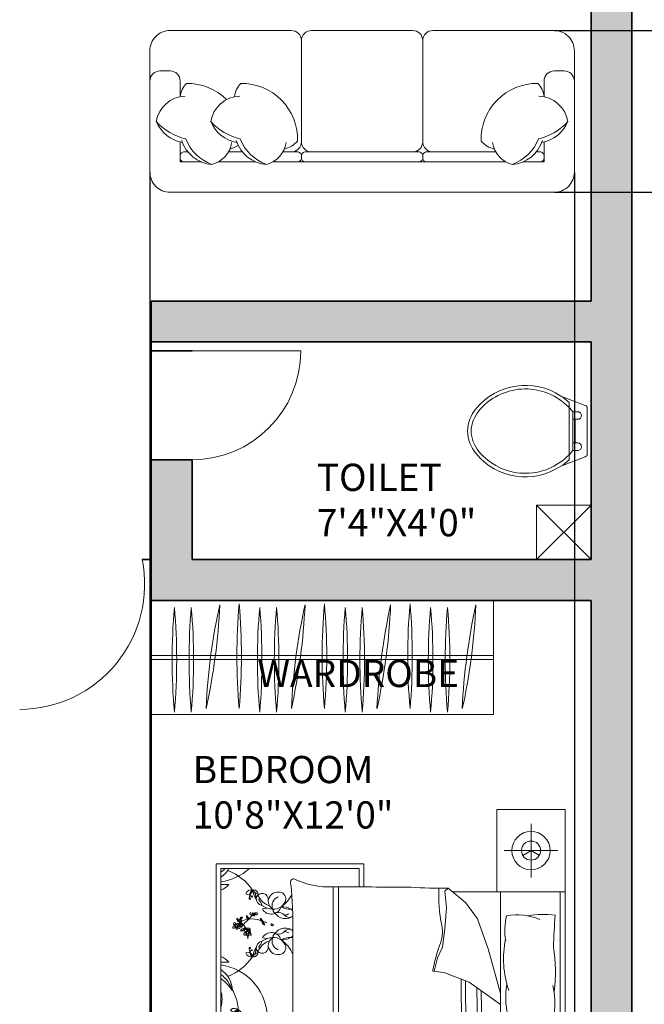
# Model space of a CAD drawing. Units: inches. Extents: x 37 to 706, y -568 to 110.
# Tile 8 of 24: x 223 to 361, y -450 to -233. Entities that reach past the tile are written whole.
import ezdxf

# ---------------------------------------------------------------- set-up
doc = ezdxf.new("R2010")
doc.units = ezdxf.units.IN
doc.header["$MEASUREMENT"] = 0
for name, color, linetype, lineweight in [('A-ANNO-DIMS', 2, 'Continuous', 18), ('A-ANNO-TEXT', 7, 'Continuous', 18), ('A-AREA-IDEN', 7, 'Continuous', 18), ('A-DOOR', 4, 'Continuous', 18), ('A-FLOR-CASE', 9, 'Continuous', 18), ('A-FLOR-FIXT', 9, 'Continuous', 18), ('A-FLOR-OPEN', 8, 'Continuous', 13), ('A-FURN', 8, 'Continuous', 13), ('A-WALL', 7, 'Continuous', 35), ('A-WALL-PATT', 252, 'Continuous', 13)]:
    doc.layers.add(name, color=color, linetype=linetype, lineweight=lineweight)
doc.styles.get("Standard").update_dxf_attribs({"font": 'arial.ttf'})
doc.dimstyles.get("Standard").update_dxf_attribs({"dimtxt": 0.18, "dimasz": 0.18, "dimexe": 0.18, "dimexo": 0.0625, "dimgap": 0.09, "dimtad": 0, "dimtih": 1, "dimtoh": 1, "dimdec": 0, "dimzin": 0, "dimdsep": 46, "dimlunit": 3, "dimtxsty": 'Standard', "dimcen": 0.09, "dimadec": 0, "dimazin": 0, "dimtfac": 1, "dimtdec": 0, "dimtofl": 0, "dimtmove": 0, "dimatfit": 3, "dimfxl": 1, "dimtolj": 1, "dimtzin": 0, "dimarcsym": 0})

# ---------------------------------------------------------------- blocks, each defined once
blk = doc.blocks.new('WARDROBE-DOUBLE')
for p, q in [((75.49, 25.16), (0, 25.16)), ((0, 25.16), (0, 0)), ((75.49, 25.16), (75.49, 0)), ((75.49, 13), (0, 13)), ((75.49, 12.16), (0, 12.16)), ((75.49, 0), (0, 0))]:
    blk.add_line(p, q)
for centre, start, end in [((-117.16, 29.99), 347.508, 357.5023), ((144.38, -4.42), 167.508, 177.5023), ((151.29, 12.89), 175.0028, 184.9972), ((-112.5, 12.89), 355.0028, 4.9972), ((-98.35, 29.99), 347.508, 357.5023), ((163.19, -4.42), 167.508, 177.5023), ((170.1, 12.89), 175.0028, 184.9972), ((-93.69, 12.89), 355.0028, 4.9972), ((182.06, -4.42), 167.508, 177.5023), ((-79.47, 29.99), 347.508, 357.5023), ((188.97, 12.89), 175.0028, 184.9972), ((-74.82, 12.89), 355.0028, 4.9972), ((200.87, -4.42), 167.508, 177.5023), ((-60.66, 29.99), 347.508, 357.5023), ((137.01, 12.08), 175.0028, 184.9972), ((-126.78, 12.08), 355.0028, 4.9972), ((140.74, 12.08), 175.0028, 184.9972), ((-123.05, 12.08), 355.0028, 4.9972), ((155.82, 12.08), 175.0028, 184.9972), ((-107.97, 12.08), 355.0028, 4.9972), ((159.55, 12.08), 175.0028, 184.9972), ((-104.24, 12.08), 355.0028, 4.9972), ((174.7, 12.08), 175.0028, 184.9972), ((-89.09, 12.08), 355.0028, 4.9972), ((178.43, 12.08), 175.0028, 184.9972), ((-85.36, 12.08), 355.0028, 4.9972), ((193.51, 12.08), 175.0028, 184.9972), ((-70.28, 12.08), 355.0028, 4.9972), ((197.24, 12.08), 175.0028, 184.9972), ((-66.55, 12.08), 355.0028, 4.9972)]:
    blk.add_arc(centre, 132.4, start, end)
blk = doc.blocks.new('WC-PLAN')
for p, q in [((22.41, 16.39), (22.41, 15.28)), ((22.41, 15.28), (22.41, 10.09)), ((22.41, 4.89), (22.41, 10.09)), ((22.41, 4.89), (22.41, 3.79))]:
    blk.add_line(p, q)
for points in [[(20.6, 17.82, 0.383919), (1.9, 15.05, 0.163732), (0, 10.09, 0.359733)], [(21.87, 15.81, 0.431639), (2.51, 14.55, 0.162618), (0.79, 10.09, 0.470877)], [(22.41, 16.39, 0.040937), (20.6, 17.82, 0.163732)], [(26.41, 10.09), (26.41, 15.13, 0.31031), (25.98, 15.75), (20.6, 17.82, 0.209071)], [(22.41, 15.28, 0.014165), (21.87, 15.81, 0.162618)], [(23.21, 14.37, 0.022712), (22.41, 15.28, 0.162618)], [(23.21, 10.09), (23.21, 14.37, 0.022712)], [(23.21, 14.37), (24.32, 14.37, -1), (24.32, 12.69), (23.74, 12.69)], [(20.6, 2.36, -0.383919), (1.9, 5.12, -0.163732), (0, 10.09, -0.359733)], [(22.41, 4.89, -0.448546), (2.51, 5.63, -0.162618), (0.79, 10.09, -0.470877)], [(26.41, 10.09), (26.41, 5.05, -0.31031), (25.98, 4.43), (20.6, 2.36, -0.209071)], [(23.21, 10.09), (23.21, 5.8, -0.476108)], [(23.21, 5.8), (24.32, 5.8, 1), (24.32, 7.49), (23.74, 7.49)], [(23.21, 5.8, -0.022712), (22.41, 4.89, -0.162618)], [(22.41, 3.79, -0.040937), (20.6, 2.36, -0.163732)]]:
    blk.add_lwpolyline(points, format="xyb")
for points in [[(23.74, 12.69), (23.21, 12.69)], [(23.74, 7.49), (23.74, 12.69)], [(23.74, 7.49), (23.21, 7.49)]]:
    blk.add_lwpolyline(points)
blk = doc.blocks.new('BED-DOUBLE-WITH-NIGHTSTANDS')
for p, q in [((77.02, 90.57), (77.02, 0)), ((69.47, 75.59), (69.47, 87.43)), ((63.56, 81.51), (75.39, 81.51)), ((0, 78.61), (32.62, 78.61)), ((0, 12.59), (0, 78.61)), ((32.62, 78.61), (32.62, 73.49)), ((1.05, 77.56), (1.05, 13.64)), ((31.58, 77.56), (1.05, 77.56)), ((31.58, 73.49), (31.58, 77.56)), ((25.85, 17.62), (25.85, 73.5)), ((26.98, 17.7), (26.98, 73.5)), ((50.48, 72.53), (51.22, 73.26)), ((50.85, 68.86), (50.48, 72.53)), ((51.22, 73.26), (55.07, 69.96)), ((77.02, 72.45), (52.16, 72.45)), ((62.71, 72.45), (62.71, 18.11)), ((75.86, 18.11), (75.86, 72.45)), ((55.07, 69.96), (57.63, 66.48)), ((10.23, 68.64), (11.25, 68.84)), ((50.48, 64.28), (50.85, 68.86)), ((57.63, 66.48), (60.02, 59.87)), ((16.95, 26.9), (16.95, 63.67)), ((49.93, 60.24), (50.48, 64.28)), ((10.23, 62.31), (11.25, 62.11)), ((48.83, 57.86), (49.93, 60.24)), ((60.02, 59.87), (62.71, 50)), ((48.1, 54.92), (48.83, 57.86)), ((50.48, 54.55), (48.1, 54.92)), ((55.8, 52.54), (50.48, 54.55)), ((54.24, 18.43), (54.09, 53.18)), ((55.17, 18.44), (55.03, 52.83)), ((62.71, 47.57), (55.8, 52.54)), ((58.02, 18.39), (57.55, 51.28)), ((58.95, 18.36), (58.49, 50.6)), ((10.23, 28.89), (11.25, 29.09)), ((10.23, 22.56), (11.25, 22.36)), ((31.58, 13.64), (31.58, 17.63)), ((32.62, 17.61), (32.62, 12.59)), ((1.05, 13.64), (31.58, 13.64)), ((69.47, 14.97), (69.47, 3.14)), ((32.62, 12.59), (0, 12.59))]:
    blk.add_line(p, q)
for points in [[(61.93, 72.45), (61.93, 90.57), (77.02, 90.57)], [(69.47, 81.51), (67.64, 80.45)], [(69.47, 81.51), (71.3, 80.45)], [(77.02, 18.11), (61.93, 18.11), (61.93, 0), (77.02, 0)], [(69.47, 9.06), (67.64, 10.11)], [(69.47, 9.06), (71.3, 10.11)]]:
    blk.add_lwpolyline(points)
for points in [[(42.92, 73.45, 0.001242), (25.74, 73.5, -0.127202), (17.18, 75.31)], [(74.76, 67.25, 0.074897), (68.85, 67.14, -0.472817)], [(68.52, 45.71, 0.14099), (74.55, 45.53, 0.235245)], [(68.52, 41.84, -0.14099), (74.55, 42.02, -0.235245)], [(74.76, 23.32, -0.074897), (68.85, 23.42, 0.472817)], [(27.69, 17.73, 0.056112), (22.71, 17.07, 0.095341), (17.91, 15.8)]]:
    blk.add_lwpolyline(points, format="xyb")
for centre, radius in [((69.47, 81.51), 4.23), ((69.47, 81.51), 2.11), ((4.52, 64.91), 0.231), ((6.95, 63.41), 0.231), ((4.52, 26.28), 0.231), ((6.95, 27.79), 0.231), ((69.47, 9.06), 4.23), ((69.47, 9.06), 2.11)]:
    blk.add_circle(centre, radius)
for centre, radius, start, end in [((-3.2, 82.51), 7.18, 306.3036, 316.4814), ((-2.13, 80.43), 5.76, 303.4617, 330.1116), ((-0.54, 86.37), 11.83, 277.745, 311.8856), ((-1.71, 66.13), 11.83, 34.3865, 68.5908), ((-0.79, 77.21), 4.81, 292.5547, 318.9546), ((1.79, 90.38), 16.36, 267.4081, 273.6519), ((17.23, 74.48), 0.836, 93.98, 207.3412), ((-77.32, 64.75), 94.28, 359.3433, 5.6887), ((7.77, 71.53), 1.31, 77.7115, 159.0387), ((7.06, 72.84), 0.988, 238.4633, 358.2869), ((10.3, 70.85), 2.99, 138.8402, 177.9352), ((8.5, 71.96), 0.967, 117.6827, 223.7762), ((8.28, 71.86), 0.98, 2.9516, 103.728), ((16.12, 74.61), 8.27, 192.5173, 207.1824), ((6.95, 71.3), 1.87, 345.4653, 54.2343), ((9.77, 73.87), 2.02, 211.3827, 255.2969), ((10.16, 70.71), 1.36, 350.264, 160.8688), ((8.69, 70.99), 0.833, 333.9755, 53.2681), ((13.65, 70.21), 2.16, 84.9449, 172.8857), ((13.86, 70.84), 1.53, 354.4856, 91.0538), ((10.57, 74.83), 6.85, 303.6671, 333.2997), ((48.97, 156.3), 83.07, 265.8294, 271.553), ((83.29, 71.71), 34.18, 177.4519, 191.3392), ((7.46, 70.95), 0.147, 177.9352, 11.4834), ((7.53, 70.96), 0.0713, 11.4834, 127.9409), ((7.89, 71.38), 0.128, 223.7762, 159.7183), ((10.57, 71.04), 1.7, 175.969, 254.3045), ((8.31, 69.21), 1.81, 6.1662, 51.5825), ((13.15, 73.4), 4.28, 211.2614, 251.7045), ((14.13, 70.59), 2.63, 182.3591, 234.0401), ((14.47, 69.36), 2.1, 111.5819, 201.4221), ((12.73, 71.31), 2.72, 265.2933, 346.921), ((1.34, 72.69), 8.6, 313.1541, 322.0459), ((7.66, 67.53), 0.177, 142.4737, 265.053), ((7.89, 67.56), 0.381, 127.7621, 169.0403), ((7.69, 67.89), 0.536, 265.053, 338.3618), ((8.4, 67.15), 0.7, 113.4276, 137.6104), ((8.32, 67.88), 0.231, 183.2768, 356.7232), ((8.49, 67.46), 0.377, 139.7889, 227.6792), ((8.37, 67.33), 0.199, 227.6792, 350.3487), ((7.6, 67.46), 0.755, 353.0852, 15.7171), ((8.1, 67.37), 0.477, 350.3487, 43.6538), ((8.98, 67.87), 0.555, 198.7263, 262.5032), ((8.54, 67.61), 0.22, 1.1081, 91.8675), ((8.68, 67.56), 0.385, 11.5637, 52.6358), ((8.95, 67.49), 0.178, 255.2356, 54.9248), ((12.81, 73.44), 4.86, 236.2883, 266.5076), ((12.18, 69.76), 2.25, 209.9085, 343.1337), ((13.13, 68.34), 0.562, 167.3041, 285.1471), ((14.65, 65.65), 3.49, 122.7011, 126.3445), ((15.31, 69.41), 2.89, 199.2822, 299.1751), ((13.76, 66), 1.86, 41.5653, 105.1471), ((16.28, 72.32), 3.75, 238.8218, 279.1554), ((14.65, 65.65), 3.49, 55.785, 94.7304), ((14.78, 69.85), 2.6, 277.436, 299.9149), ((15.95, 67.67), 1.09, 30.0293, 52.325), ((66.47, 55.71), 11.67, 65.1316, 101.7583), ((4.34, 65.38), 0.455, 157.4086, 261.4386), ((4.09, 65.4), 0.229, 58.0499, 135.6268), ((4.32, 65.26), 0.153, 172.906, 277.132), ((3.82, 64.98), 0.727, 14.7558, 58.0499), ((4.84, 65.17), 0.315, 36.1046, 181.4281), ((4.85, 66.4), 0.258, 124.3538, 214.3923), ((5.23, 66.36), 0.6, 190.3057, 287.1958), ((4.66, 65.42), 0.317, 270.0645, 331.1507), ((5.41, 66.58), 0.697, 176.9701, 248.2913), ((10.38, 70.25), 6.74, 212.6784, 216.3746), ((4.92, 65.2), 0.226, 263.7526, 41.7054), ((5.17, 66.41), 0.267, 216.3746, 291.7548), ((7.53, 62.67), 3.76, 124.0033, 132.4917), ((3.66, 62.2), 4.02, 63.7819, 68.2913), ((5.81, 65.29), 0.639, 128.3208, 208.8162), ((5.81, 66.23), 0.6, 122.8155, 187.3992), ((5.34, 65.98), 0.201, 289.3605, 111.7548), ((5.49, 65.98), 0.201, 221.8703, 44.2646), ((6.41, 65.39), 1.05, 157.2305, 229.0635), ((6.07, 66.15), 0.697, 109.4799, 177.6828), ((6.05, 65.74), 0.619, 174.4544, 220.6188), ((2.53, 62.29), 4.51, 30.544, 49.818), ((5.7, 66.59), 0.258, 56.8636, 146.9021), ((5.83, 66.31), 0.267, 148.8844, 224.2646), ((5.02, 64.86), 0.744, 340.0041, 40.6188), ((11.37, 62.96), 6.74, 145.1882, 148.8844), ((7.53, 62.67), 3.76, 94.756, 119.2041), ((15.54, 57.26), 12.37, 132.2412, 142.1744), ((9.29, 67.11), 2.55, 178.3264, 187.1302), ((6.53, 66.75), 0.476, 11.3256, 64.4621), ((8.15, 67.44), 1.43, 190.2588, 210.656), ((7.19, 66.85), 0.435, 188.3432, 274.2869), ((7.57, 67.09), 0.759, 210.656, 242.6341), ((8.14, 67.75), 1.46, 218.2101, 226.3071), ((7.07, 66.52), 0.185, 325.7657, 67.4417), ((7.72, 58.94), 7.5, 73.5842, 93.8277), ((12.34, 66.57), 2.55, 178.3264, 187.1302), ((9.58, 66.21), 0.476, 11.3256, 64.4621), ((11.19, 66.9), 1.43, 190.2588, 210.656), ((10.23, 66.31), 0.435, 188.3432, 274.2869), ((10.61, 66.55), 0.759, 210.656, 242.6341), ((11.19, 67.21), 1.46, 218.2101, 226.3071), ((10.11, 65.98), 0.185, 325.7657, 67.4417), ((10.63, 65.65), 0.435, 147.5332, 233.4768), ((11.02, 65.87), 0.759, 179.1859, 211.164), ((10.28, 65.7), 0.185, 354.3784, 96.0543), ((7.72, 58.94), 7.5, 63.0032, 69.8941), ((11.6, 66.22), 1.43, 211.164, 231.5612), ((11.85, 67.38), 2.55, 234.6898, 243.4936), ((11.87, 66.07), 1.46, 195.5129, 203.6099), ((10.23, 65.12), 0.476, 357.3579, 50.4944), ((12.28, 65.21), 0.175, 12.7051, 190.4384), ((12.38, 65.23), 0.284, 190.4384, 10.4136), ((16.16, 68.13), 1.36, 221.5653, 293.8354), ((15.95, 67.67), 1.09, 314.4517, 333.558), ((75.82, 64.02), 12.14, 165.1039, 191.0369), ((936.66, 17.33), 863.34, 176.68521, 177.14978), ((3.86, 64.56), 0.177, 142.4737, 265.053), ((4.09, 64.6), 0.381, 61.2196, 169.0403), ((3.89, 64.92), 0.536, 265.053, 338.3618), ((4.6, 64.19), 0.7, 113.4276, 137.6104), ((4.69, 64.5), 0.377, 139.7889, 227.6792), ((4.57, 64.37), 0.199, 227.6792, 350.3487), ((3.8, 64.5), 0.755, 353.0852, 15.7171), ((4.29, 64.41), 0.477, 350.3487, 43.6538), ((5.18, 64.9), 0.555, 198.7263, 262.5032), ((4.93, 65.34), 0.363, 221.8413, 265.7877), ((4.74, 64.65), 0.22, 1.1081, 91.8675), ((4.88, 64.6), 0.385, 11.5637, 86.365), ((5.15, 64.53), 0.178, 255.2356, 54.9248), ((5.92, 65.34), 0.764, 207.7043, 254.3516), ((5.43, 64.9), 1.05, 270.278, 342.111), ((6.13, 63.58), 0.744, 98.7227, 159.3375), ((5.75, 64.54), 0.764, 244.9899, 291.6373), ((5.92, 64.93), 0.619, 278.7227, 324.8872), ((5.81, 64.43), 0.639, 290.5253, 358.5375), ((6.29, 63.06), 0.177, 142.4737, 265.053), ((6.52, 63.09), 0.381, 61.2196, 169.0403), ((6.32, 63.41), 0.536, 265.053, 338.3618), ((6.77, 63.88), 0.455, 157.4086, 261.4386), ((6.52, 63.89), 0.229, 58.0499, 135.6268), ((7.06, 64.61), 0.639, 182.8499, 266.1226), ((6.81, 65.06), 0.619, 231.7607, 277.9252), ((7.29, 65.17), 1.05, 214.5369, 286.3699), ((7.03, 62.68), 0.7, 113.4276, 137.6104), ((6.76, 63.75), 0.153, 172.906, 277.132), ((6.25, 63.47), 0.727, 14.7558, 58.0499), ((2.53, 62.29), 4.51, 23.0501, 23.8477), ((7.12, 62.99), 0.377, 139.7889, 227.6792), ((7, 63.71), 0.744, 37.3105, 97.9252), ((7.27, 63.66), 0.315, 36.1046, 181.4281), ((6.23, 62.99), 0.755, 353.0852, 15.7171), ((7.08, 64.73), 0.764, 265.0106, 311.658), ((6.72, 62.9), 0.477, 350.3487, 43.6538), ((7.61, 63.4), 0.555, 198.7263, 262.5032), ((7.09, 63.91), 0.317, 270.0645, 331.1507), ((7.36, 63.83), 0.363, 221.8413, 265.7877), ((7.17, 63.14), 0.22, 1.1081, 91.8675), ((7.36, 63.7), 0.226, 263.7526, 41.7054), ((7.31, 63.09), 0.385, 11.5637, 86.365), ((7.58, 63.02), 0.178, 255.2356, 54.9248), ((12.18, 61.19), 2.25, 16.8663, 150.0915), ((13.13, 62.61), 0.562, 74.8529, 192.6959), ((15.31, 61.54), 2.89, 60.8249, 160.7178), ((13.76, 64.95), 1.86, 254.8529, 318.4347), ((14.78, 61.1), 2.6, 60.0851, 82.564), ((16.16, 62.82), 1.36, 66.1646, 138.4347), ((15.95, 63.28), 1.09, 23.229, 45.5483), ((42.55, 63.54), 7.37, 336.2616, 11.3392), ((7, 62.86), 0.199, 227.6792, 350.3487), ((2.53, 62.29), 4.51, 357.1071, 4.7585), ((10.57, 59.91), 1.7, 105.6955, 184.031), ((8.31, 61.74), 1.81, 308.4175, 353.8338), ((13.15, 57.54), 4.28, 108.2955, 148.7386), ((12.81, 57.5), 4.86, 93.4924, 123.7117), ((14.13, 60.36), 2.63, 125.9599, 177.6409), ((14.47, 61.59), 2.1, 158.5779, 248.4181), ((12.73, 59.64), 2.72, 13.079, 94.7067), ((14.65, 65.3), 3.49, 233.6555, 237.2989), ((16.28, 58.63), 3.75, 79.7133, 121.1782), ((14.65, 65.3), 3.49, 265.2696, 304.215), ((10.57, 56.11), 6.85, 21.4941, 56.3329), ((15.95, 63.28), 1.09, 307.675, 336.7144), ((84.45, 57.63), 21.05, 168.0397, 199.2615), ((7.06, 58.1), 0.988, 1.7131, 121.5367), ((7.77, 59.41), 1.31, 200.9613, 282.2885), ((7.46, 60), 0.147, 348.5166, 182.0648), ((10.3, 60.1), 2.99, 182.0648, 221.1598), ((7.53, 59.98), 0.0713, 232.0591, 348.5166), ((8.5, 58.99), 0.967, 136.2238, 242.3173), ((7.94, 59.56), 0.0771, 200.2667, 136.2271), ((6.95, 59.65), 1.87, 305.7657, 14.5347), ((16.12, 56.34), 8.27, 152.8176, 167.4827), ((8.28, 59.09), 0.98, 256.272, 357.0484), ((9.77, 57.08), 2.02, 104.7031, 148.6173), ((10.16, 60.24), 1.36, 199.1312, 9.736), ((8.69, 59.96), 0.833, 306.7319, 26.0245), ((13.65, 60.74), 2.16, 187.1143, 275.0551), ((13.86, 60.11), 1.53, 268.9462, 5.5144), ((82.33, 48.63), 35.12, 160.1194, 169.3383), ((41.99, 54.84), 32.85, 352.2196, 9.497), ((-0.79, 53.74), 4.81, 41.0454, 67.4453), ((1.79, 40.57), 16.36, 86.3481, 92.5919), ((-1.71, 64.81), 11.83, 291.4092, 325.6135), ((-0.54, 44.58), 11.83, 4.4623, 82.255), ((-2.13, 50.51), 5.76, 1.272, 56.5383), ((48.03, 55.13), 0.219, 178.8623, 289.7536), ((-3.2, 48.44), 7.18, 17.8504, 53.6964), ((-5.22, 44.66), 10.68, 34.0123, 54.053), ((-5.17, 48.79), 6.5, 343.5431, 17.0202), ((-6.88, 45.48), 11.83, 4.4623, 27.4146), ((79.85, 49.11), 15.97, 169.8617, 193.6238), ((58.59, 47.9), 16.14, 351.5249, 13.96), ((-8.52, 46.22), 9.62, 4.3787, 5.6357), ((-15.11, 41.15), 17.18, 19.7217, 19.9028), ((4.03, 45.43), 1.31, 47.7873, 129.1145), ((4.07, 46.92), 0.988, 208.5391, 328.3627), ((5.88, 43.58), 2.99, 108.9159, 148.011), ((4.87, 45.44), 0.967, 87.7585, 193.852), ((12.81, 43.93), 8.27, 162.593, 177.2582), ((3.21, 45.64), 1.87, 315.5411, 24.3101), ((6.93, 46.46), 2.02, 181.4585, 225.3727), ((4.64, 45.46), 0.98, 333.0274, 73.8037), ((10.37, 44.53), 1.31, 47.7873, 129.1145), ((65.49, 56.38), 11.1, 264.0129, 285.8293), ((3.47, 45.08), 0.147, 148.011, 341.5592), ((3.54, 45.06), 0.0713, 341.5592, 98.0167), ((4.06, 45.24), 0.128, 193.852, 129.9245), ((12.81, 44.25), 8.27, 182.7418, 197.407), ((3.21, 42.54), 1.87, 335.6899, 44.4589), ((10.41, 46.02), 0.988, 208.5391, 328.3627), ((9.8, 44.18), 0.147, 148.011, 341.5592), ((9.8, 44), 0.147, 18.4408, 211.989), ((12.22, 42.67), 2.99, 108.9159, 148.011), ((12.22, 45.51), 2.99, 211.989, 251.0841), ((9.88, 44.15), 0.0713, 341.5592, 98.0167), ((9.88, 44.03), 0.0713, 261.9833, 18.4408), ((11.21, 44.53), 0.967, 87.7585, 193.852), ((11.21, 43.65), 0.967, 166.148, 272.2415), ((10.39, 44.33), 0.128, 193.852, 129.9245), ((10.44, 43.86), 0.0771, 230.1909, 166.0209), ((9.54, 44.73), 1.87, 315.5411, 24.3101), ((19.14, 43.02), 8.27, 162.593, 177.2582), ((9.54, 43.45), 1.87, 335.6899, 44.4589), ((19.14, 45.16), 8.27, 182.7418, 197.407), ((10.97, 44.56), 0.98, 333.0274, 73.8037), ((13.27, 45.55), 2.02, 181.4585, 225.3727), ((10.97, 43.62), 0.98, 286.1963, 26.9726), ((13.27, 42.63), 2.02, 134.6273, 178.5415), ((2.19, 43.98), 9.15, 262.8636, 351.8197), ((4.07, 41.26), 0.988, 31.6373, 151.4609), ((4.03, 42.75), 1.31, 230.8855, 312.2127), ((3.47, 43.1), 0.147, 18.4408, 211.989), ((5.88, 44.6), 2.99, 211.989, 251.0841), ((3.54, 43.12), 0.0713, 261.9833, 18.4408), ((-6.88, 42.69), 11.83, 332.5854, 355.5377), ((4.87, 42.74), 0.967, 166.148, 272.2415), ((4.11, 42.95), 0.0771, 230.1909, 166.0209), ((6.93, 41.72), 2.02, 134.6273, 178.5415), ((4.64, 42.72), 0.98, 286.1963, 26.9726), ((10.41, 42.16), 0.988, 31.6373, 151.4609), ((10.37, 43.65), 1.31, 230.8855, 312.2127), ((68.68, 40.17), 4.8, 155.0183, 198.5407), ((65.49, 31.16), 11.1, 74.1707, 95.9871), ((70.25, 40.78), 4.48, 333.3437, 16.1026), ((-5.17, 39.39), 6.5, 342.9798, 16.4569), ((-8.52, 41.96), 9.62, 354.3643, 355.6213), ((-15.11, 47.03), 17.18, 340.0972, 340.2783), ((3.02, 42.8), 5.3, 248.117, 276.6195), ((1.55, 37.94), 2.12, 256.3898, 349.0739), ((1.84, 39.54), 2.68, 252.8609, 311.9049), ((-1.71, 26.39), 11.83, 34.3865, 68.5908), ((58.92, 34.06), 15.92, 346.3427, 11.1841), ((74.93, 31.78), 11.53, 153.8761, 196.1746), ((1.79, 50.63), 16.36, 267.4081, 273.6519), ((-0.79, 37.46), 4.81, 292.5547, 318.9546), ((7.77, 31.78), 1.31, 77.7115, 159.0387), ((7.06, 33.09), 0.988, 238.4633, 358.2869), ((10.3, 31.1), 2.99, 138.8402, 177.9352), ((8.5, 32.21), 0.967, 117.6827, 223.7762), ((8.28, 32.11), 0.98, 2.9516, 103.728), ((9.77, 34.12), 2.02, 211.3827, 255.2969), ((6.95, 31.55), 1.87, 345.4653, 54.2343), ((16.12, 34.86), 8.27, 192.5173, 207.1824), ((13.65, 30.46), 2.16, 84.9449, 172.8857), ((13.86, 31.09), 1.53, 354.4856, 91.0538), ((10.57, 35.08), 6.85, 303.6671, 338.5059), ((7.46, 31.2), 0.147, 177.9352, 11.4834), ((7.53, 31.21), 0.0713, 11.4834, 127.9409), ((7.89, 31.63), 0.128, 223.7762, 159.7183), ((10.16, 30.96), 1.36, 350.264, 160.8688), ((10.57, 31.29), 1.7, 175.969, 254.3045), ((8.69, 31.24), 0.833, 333.9755, 53.2681), ((8.31, 29.46), 1.81, 6.1662, 51.5825), ((13.15, 33.66), 4.28, 211.2614, 251.7045), ((14.13, 30.84), 2.63, 182.3591, 234.0401), ((14.47, 29.61), 2.1, 111.5819, 201.4221), ((12.73, 31.56), 2.72, 265.2933, 346.921), ((6.29, 28.14), 0.177, 94.947, 217.5263), ((6.32, 27.78), 0.536, 21.6382, 94.947), ((7.12, 28.21), 0.377, 132.3208, 220.2111), ((7, 28.34), 0.199, 9.6513, 132.3208), ((6.23, 28.2), 0.755, 344.2829, 6.9148), ((2.53, 28.91), 4.51, 355.2415, 2.8929), ((6.72, 28.3), 0.477, 316.3462, 9.6513), ((7.61, 27.8), 0.555, 97.4968, 161.2737), ((7.58, 28.18), 0.178, 305.0752, 104.7644), ((12.81, 33.7), 4.86, 236.2883, 266.5076), ((12.18, 30.01), 2.25, 209.9085, 343.1337), ((13.13, 28.59), 0.562, 167.3041, 285.1471), ((14.65, 25.9), 3.49, 122.7011, 126.3445), ((15.31, 29.66), 2.89, 199.2822, 299.1751), ((16.28, 32.57), 3.75, 238.8218, 280.2867), ((14.65, 25.9), 3.49, 55.785, 94.7304), ((15.95, 27.92), 1.09, 23.2856, 52.325), ((75.82, 26.55), 12.14, 168.9631, 194.8961), ((936.66, 73.23), 863.34, 182.85022, 183.31479), ((3.86, 26.63), 0.177, 94.947, 217.5263), ((4.09, 26.6), 0.381, 190.9597, 298.7804), ((3.89, 26.28), 0.536, 21.6382, 94.947), ((4.34, 25.81), 0.455, 98.5614, 202.5914), ((4.6, 27.01), 0.7, 222.3896, 246.5724), ((4.32, 25.94), 0.153, 82.868, 187.094), ((4.69, 26.7), 0.377, 132.3208, 220.2111), ((4.57, 26.83), 0.199, 9.6513, 132.3208), ((3.8, 26.7), 0.755, 344.2829, 6.9148), ((4.29, 26.79), 0.477, 316.3462, 9.6513), ((5.18, 26.29), 0.555, 97.4968, 161.2737), ((4.93, 25.86), 0.363, 94.2123, 138.1587), ((4.66, 25.78), 0.317, 28.8493, 89.9355), ((4.74, 26.55), 0.22, 268.1325, 358.8919), ((4.88, 26.6), 0.385, 273.635, 348.4363), ((4.92, 25.99), 0.226, 318.2946, 96.2474), ((5.15, 26.67), 0.178, 305.0752, 104.7644), ((5.81, 25.91), 0.639, 151.1838, 231.6792), ((5.92, 25.86), 0.764, 105.6484, 152.2957), ((6.41, 25.8), 1.05, 130.9365, 202.7695), ((5.75, 26.66), 0.764, 68.3627, 115.0101), ((5.43, 26.3), 1.05, 17.889, 89.722), ((6.13, 27.61), 0.744, 200.6625, 261.2773), ((2.53, 28.91), 4.51, 310.182, 329.456), ((5.02, 26.34), 0.744, 319.3812, 19.9959), ((15.54, 33.94), 12.37, 217.8256, 227.7588), ((5.92, 26.27), 0.619, 35.1128, 81.2773), ((5.81, 26.77), 0.639, 1.4625, 69.4747), ((6.52, 28.11), 0.381, 190.9597, 298.7804), ((6.77, 27.32), 0.455, 98.5614, 202.5914), ((6.52, 27.31), 0.229, 224.3732, 301.9501), ((7.06, 26.59), 0.639, 93.8774, 177.1501), ((7.29, 26.03), 1.05, 73.6301, 145.4631), ((6.81, 26.14), 0.619, 82.0748, 128.2393), ((7.03, 28.52), 0.7, 222.3896, 246.5724), ((6.76, 27.45), 0.153, 82.868, 187.094), ((6.25, 27.73), 0.727, 301.9501, 345.2442), ((2.53, 28.91), 4.51, 336.1523, 336.9499), ((7, 27.49), 0.744, 262.0748, 322.6895), ((7.27, 27.54), 0.315, 178.5719, 323.8954), ((7.08, 26.46), 0.764, 48.342, 94.9894), ((7.36, 27.37), 0.363, 94.2123, 138.1587), ((7.09, 27.29), 0.317, 28.8493, 89.9355), ((7.17, 28.06), 0.22, 268.1325, 358.8919), ((7.31, 28.11), 0.385, 273.635, 348.4363), ((7.36, 27.5), 0.226, 318.2946, 96.2474), ((11.6, 24.98), 1.43, 128.4388, 148.836), ((11.85, 23.82), 2.55, 116.5064, 125.3102), ((10.23, 26.08), 0.476, 309.5056, 2.6421), ((12.38, 25.96), 0.284, 349.5864, 169.5616), ((13.76, 26.25), 1.86, 41.5653, 105.1471), ((14.78, 30.1), 2.6, 277.436, 299.9149), ((16.16, 28.38), 1.36, 221.5653, 293.8354), ((-71.13, 24.12), 88.13, 355.2402, 1.8035), ((15.95, 27.92), 1.09, 314.4517, 336.7144), ((4.09, 25.8), 0.229, 224.3732, 301.9501), ((3.82, 26.22), 0.727, 301.9501, 345.2442), ((4.84, 26.03), 0.315, 178.5719, 323.8954), ((4.85, 24.8), 0.258, 145.6077, 235.6462), ((5.23, 24.83), 0.6, 72.8042, 169.6943), ((5.41, 24.62), 0.697, 111.7087, 183.0299), ((10.38, 20.95), 6.74, 143.6254, 147.3216), ((5.17, 24.78), 0.267, 68.2452, 143.6254), ((7.53, 28.53), 3.76, 227.5083, 235.9967), ((3.66, 29), 4.02, 291.7087, 296.2181), ((5.81, 24.97), 0.6, 172.6008, 237.1845), ((5.34, 25.22), 0.201, 248.2452, 70.6395), ((5.49, 25.22), 0.201, 315.7354, 138.1297), ((6.07, 25.05), 0.697, 182.3172, 250.5201), ((6.05, 25.46), 0.619, 139.3812, 185.5456), ((5.7, 24.61), 0.258, 213.0979, 303.1364), ((5.83, 24.89), 0.267, 135.7354, 211.1156), ((11.37, 28.24), 6.74, 211.1156, 214.8118), ((7.53, 28.53), 3.76, 240.7959, 265.244), ((8.15, 23.76), 1.43, 149.344, 169.7412), ((9.29, 24.09), 2.55, 172.8698, 181.6736), ((6.53, 24.45), 0.476, 295.5379, 348.6744), ((7.19, 24.34), 0.435, 85.7131, 171.6568), ((7.57, 24.1), 0.759, 117.3659, 149.344), ((8.14, 23.45), 1.46, 133.6929, 141.7899), ((7.07, 24.67), 0.185, 292.5583, 34.2343), ((7.72, 32.26), 7.5, 266.1723, 286.4158), ((1.34, 18.5), 8.6, 37.9541, 46.8459), ((8.49, 23.74), 0.377, 132.3208, 220.2111), ((8.37, 23.87), 0.199, 9.6513, 132.3208), ((8.1, 23.82), 0.477, 316.3462, 9.6513), ((8.98, 23.33), 0.555, 97.4968, 161.2737), ((8.95, 23.71), 0.178, 305.0752, 104.7644), ((11.19, 24.3), 1.43, 149.344, 169.7412), ((12.34, 24.63), 2.55, 172.8698, 181.6736), ((9.58, 24.98), 0.476, 295.5379, 348.6744), ((10.23, 24.88), 0.435, 85.7131, 171.6568), ((10.61, 24.64), 0.759, 117.3659, 149.344), ((11.19, 23.99), 1.46, 133.6929, 141.7899), ((10.11, 25.21), 0.185, 292.5583, 34.2343), ((10.63, 25.55), 0.435, 126.5232, 212.4668), ((11.02, 25.33), 0.759, 148.836, 180.8141), ((10.28, 25.5), 0.185, 263.9457, 5.6216), ((7.72, 32.26), 7.5, 290.1059, 296.9968), ((11.87, 25.13), 1.46, 156.3901, 164.4871), ((12.28, 25.98), 0.175, 169.5616, 347.2949), ((15.31, 21.79), 2.89, 60.8249, 160.7178), ((13.76, 25.2), 1.86, 254.8529, 318.4347), ((14.78, 21.35), 2.6, 60.0851, 82.564), ((16.16, 23.07), 1.36, 66.1646, 138.4347), ((15.95, 23.53), 1.09, 16.6343, 45.5483), ((66.47, 34.85), 11.67, 258.2417, 294.8684), ((7.66, 23.67), 0.177, 94.947, 217.5263), ((7.89, 23.64), 0.381, 190.9597, 232.2379), ((7.69, 23.31), 0.536, 21.6382, 94.947), ((8.4, 24.05), 0.7, 222.3896, 246.5724), ((8.32, 23.32), 0.231, 3.2768, 176.7232), ((7.6, 23.73), 0.755, 344.2829, 6.9148), ((8.54, 23.59), 0.22, 268.1325, 358.8919), ((10.57, 20.16), 1.7, 105.6955, 184.031), ((8.68, 23.64), 0.385, 307.3642, 348.4363), ((8.31, 21.99), 1.81, 308.4175, 353.8338), ((13.15, 17.79), 4.28, 108.2955, 148.7386), ((12.81, 17.75), 4.86, 93.4924, 123.7117), ((12.18, 21.44), 2.25, 16.8663, 150.0915), ((14.13, 20.61), 2.63, 125.9599, 177.6409), ((14.47, 21.84), 2.1, 158.5779, 248.4181), ((12.73, 19.89), 2.72, 13.079, 94.7067), ((13.13, 22.86), 0.562, 74.8529, 192.6959), ((14.65, 25.55), 3.49, 233.6555, 237.2989), ((16.28, 18.88), 3.75, 79.249, 121.1782), ((14.65, 25.55), 3.49, 265.2696, 304.215), ((10.57, 16.37), 6.85, 23.6453, 56.3329), ((15.95, 23.53), 1.09, 307.675, 342.5814), ((7.46, 20.25), 0.147, 348.5166, 182.0648), ((10.3, 20.35), 2.99, 182.0648, 221.1598), ((7.53, 20.24), 0.0713, 232.0591, 348.5166), ((8.5, 19.24), 0.967, 136.2238, 242.3173), ((7.94, 19.81), 0.0771, 200.2667, 136.2271), ((16.12, 16.59), 8.27, 152.8176, 167.4827), ((6.95, 19.9), 1.87, 305.7657, 14.5347), ((10.16, 20.49), 1.36, 199.1312, 9.736), ((8.69, 20.21), 0.833, 306.7319, 26.0245), ((13.65, 20.99), 2.16, 187.1143, 275.0551), ((13.86, 20.36), 1.53, 268.9462, 5.5144), ((-0.79, 13.99), 4.81, 41.0454, 67.4453), ((-1.71, 25.06), 11.83, 291.4092, 325.6135), ((7.06, 18.36), 0.988, 1.7131, 121.5367), ((7.77, 19.67), 1.31, 200.9613, 282.2885), ((9.77, 17.33), 2.02, 104.7031, 148.6173), ((8.28, 19.34), 0.98, 256.272, 357.0484), ((45.72, -193.78), 212.28, 89.1145, 94.8735), ((51.64, -144.24), 162.73, 86.1, 90.9282), ((1.79, 0.82), 16.36, 86.3481, 92.5919), ((-0.54, 4.83), 11.83, 48.1144, 82.255), ((-2.13, 10.76), 5.76, 29.8884, 56.5383), ((17.45, 16.48), 0.826, 156.5219, 303.8264), ((-3.2, 8.69), 7.18, 43.5186, 53.6964)]:
    blk.add_arc(centre, radius, start, end)
blk = doc.blocks.new('DOOR-SWING-24')
blk.add_line((0, 0), (0, 24))
blk.add_arc((0, 0), 24, 0, 90)
blk = doc.blocks.new('FLOOR-OPENING-12-SQ')
for p, q in [((0, 0), (0, 12)), ((0, 12), (12, 12)), ((12, 12), (0, 0)), ((12, 0), (0, 12))]:
    blk.add_line(p, q)
blk = doc.blocks.new('*D49')
at = {"layer": 'A-ANNO-DIMS', "color": 0, "lineweight": -2, "transparency": 16777216}
for p, q in [((251.66, -266.36), (251.66, -567.64)), ((345.27, -266.36), (345.27, -567.64)), ((251.84, -567.46), (297.93, -567.46)), ((345.09, -567.46), (299, -567.46))]:
    blk.add_line(p, q, dxfattribs=at)
at = {"layer": 'A-ANNO-DIMS', "color": 0, "transparency": 16777216}
for points in [[(251.84, -567.43), (251.84, -567.49), (251.66, -567.46)], [(345.09, -567.43), (345.09, -567.49), (345.27, -567.46)]]:
    blk.add_solid(points, dxfattribs=at)
at = {"layer": 'Defpoints', "color": 0, "transparency": 16777216}
for p in [(251.66, -266.29), (345.27, -266.29), (345.27, -567.46)]:
    blk.add_point(p, dxfattribs=at)
at = {"layer": 'A-ANNO-DIMS', "color": 0, "transparency": 16777216, "insert": (298.47, -567.46), "char_height": 0.18, "attachment_point": 5}
blk.add_mtext('\\A1;7\'-9 1/2"', dxfattribs=at)
blk = doc.blocks.new('*D50')
at = {"layer": 'A-ANNO-DIMS', "color": 0, "lineweight": -2, "transparency": 16777216}
for p, q in [((340.88, -235.09), (705.89, -235.09)), ((705.71, -235.27), (705.71, -252.74)), ((705.71, -270.57), (705.71, -253.1)), ((340.88, -270.75), (705.89, -270.75))]:
    blk.add_line(p, q, dxfattribs=at)
at = {"layer": 'A-ANNO-DIMS', "color": 0, "transparency": 16777216}
for points in [[(705.68, -235.27), (705.74, -235.27), (705.71, -235.09)], [(705.68, -270.57), (705.74, -270.57), (705.71, -270.75)]]:
    blk.add_solid(points, dxfattribs=at)
at = {"layer": 'Defpoints', "color": 0, "transparency": 16777216}
for p in [(340.81, -235.09), (340.81, -270.75), (705.71, -270.75)]:
    blk.add_point(p, dxfattribs=at)
at = {"layer": 'A-ANNO-DIMS', "color": 0, "transparency": 16777216, "insert": (705.71, -252.92), "char_height": 0.18, "attachment_point": 5}
blk.add_mtext('\\A1;2\'-11 1/2"', dxfattribs=at)
blk = doc.blocks.new('*D51')
at = {"layer": 'A-ANNO-DIMS', "color": 0, "lineweight": -2, "transparency": 16777216}
for p, q in [((220.96, -294.77), (220.96, -567.64)), ((251.96, -294.77), (251.96, -567.64)), ((221.14, -567.46), (236.13, -567.46)), ((251.78, -567.46), (236.79, -567.46))]:
    blk.add_line(p, q, dxfattribs=at)
at = {"layer": 'A-ANNO-DIMS', "color": 0, "transparency": 16777216}
for points in [[(221.14, -567.43), (221.14, -567.49), (220.96, -567.46)], [(251.78, -567.43), (251.78, -567.49), (251.96, -567.46)]]:
    blk.add_solid(points, dxfattribs=at)
at = {"layer": 'Defpoints', "color": 0, "transparency": 16777216}
for p in [(220.96, -294.71), (251.96, -294.71), (251.96, -567.46)]:
    blk.add_point(p, dxfattribs=at)
at = {"layer": 'A-ANNO-DIMS', "color": 0, "transparency": 16777216, "insert": (236.46, -567.46), "char_height": 0.18, "attachment_point": 5}
blk.add_mtext('\\A1;2\'-7"', dxfattribs=at)

msp = doc.modelspace()

# ---------------------------------------------------------------- hatches: boundary and pattern name
at = {"layer": 'A-WALL-PATT'}
h = msp.add_hatch(color=256, dxfattribs=at)
h.dxf.hatch_style = 1
h.paths.add_polyline_path([(220.96, -351.71), (211.96, -351.71), (211.96, -513.71), (254.96, -513.71), (254.96, -504.71), (220.96, -504.71)], flags=17)
h.paths.add_polyline_path([(220.96, -294.71), (211.96, -294.71), (211.96, -303.71), (220.96, -303.71)], flags=17)
h.paths.add_polyline_path([(175.96, -294.71), (155.87, -294.71), (155.87, -303.71), (155.96, -303.71), (175.96, -303.71)], flags=17)
h.paths.add_polyline_path([(220.96, -16.71), (211.96, -16.71), (211.96, -142.71), (220.96, -142.71)], flags=17)
h.paths.add_polyline_path([(357.96, 51.29), (78.96, 51.29), (78.96, -513.71), (87.96, -513.71), (87.96, -303.71), (95.87, -303.71), (95.87, -294.71), (87.96, -294.71), (87.96, -142.71), (187.96, -142.71), (187.96, -133.71), (87.96, -133.71), (87.96, -25.71), (106.96, -25.71), (106.96, -16.71), (87.96, -16.71), (87.96, 42.29), (348.96, 42.29), (348.96, 17.13), (348.96, -133.71), (246.96, -133.71), (246.96, -142.71), (348.96, -142.71), (348.96, -294.71), (251.96, -294.71), (251.96, -303.71), (348.96, -303.71), (348.96, -351.71), (260.96, -351.71), (260.96, -329.71), (251.96, -329.71), (251.96, -360.71), (327.45, -360.71), (348.96, -360.71), (348.96, -504.71), (314.96, -504.71), (314.96, -513.71), (357.96, -513.71)])
h.paths.add_polyline_path([(416.96, -303.71), (402.96, -303.71), (402.96, -151.71), (478.96, -151.71), (478.96, -142.71), (402.96, -142.71), (402.96, -22.71), (409.96, -22.71), (409.96, -13.71), (402.96, -13.71), (402.96, 42.29), (663.96, 42.29), (663.96, -303.71), (566.96, -303.71), (566.96, -312.71), (663.96, -312.71), (663.96, -360.71), (575.96, -360.71), (575.96, -338.71), (566.96, -338.71), (566.96, -360.71), (566.96, -369.71), (642.45, -369.71), (663.96, -369.71), (663.96, -513.71), (629.96, -513.71), (629.96, -522.71), (672.96, -522.71), (672.96, 51.29), (393.96, 51.29), (393.96, -522.71), (402.96, -522.71), (402.96, -312.71), (416.96, -312.71)])
h.paths.add_polyline_path([(490.96, -303.71), (476.96, -303.71), (476.96, -312.71), (490.96, -312.71)], flags=17)
h.paths.add_polyline_path([(535.96, -303.71), (526.96, -303.71), (526.96, -312.71), (535.96, -312.71)], flags=17)
h.paths.add_polyline_path([(535.96, -369.71), (526.96, -369.71), (526.96, -522.71), (569.96, -522.71), (569.96, -513.71), (535.96, -513.71)], flags=17)
h.paths.add_polyline_path([(511.96, -13.71), (502.96, -13.71), (502.96, -151.71), (511.96, -151.71)], flags=17)
h.paths.add_polyline_path([(651.54, -142.71), (651.54, -120.18), (642.54, -120.18), (642.54, -142.71), (550.54, -142.71), (550.54, -120.71), (541.54, -120.71), (541.54, -142.71), (537.96, -142.71), (537.96, -151.71), (651.54, -151.71)], flags=17)
h.paths.add_polyline_path([(651.54, -85.71), (541.54, -85.71), (541.54, -94.71), (651.54, -94.71)], flags=17)
h.paths.add_polyline_path([(476.96, -13.71), (469.96, -13.71), (469.96, -22.71), (476.96, -22.71)], flags=17)
h.paths.add_polyline_path([(185.96, -16.71), (166.96, -16.71), (166.96, -25.71), (185.96, -25.71)], flags=17)
h.paths.add_polyline_path([(168.91, -414.72), (214.62, -414.72), (214.62, -392.33), (168.91, -392.33)], flags=25)

# ---------------------------------------------------------------- linework, layer by layer
at = {"layer": 'A-DOOR'}
msp.add_arc((222.96, -357.16), 27.55, 270, 11.4212, dxfattribs=at)
at = {"layer": 'A-FURN', "ltscale": 0.03}
msp.add_lwpolyline([(345.27, -239.55, 0.414214), (340.81, -235.09), (314.07, -235.09, 0.414214), (311.84, -237.32, 0.414214), (309.61, -235.09), (287.32, -235.09, 0.414214), (285.09, -237.32, 0.414214), (282.86, -235.09), (256.12, -235.09, 0.414214), (251.66, -239.55), (251.66, -266.29, 0.414214), (256.12, -270.75), (340.81, -270.75, 0.414214), (345.27, -266.29)], format="xyb", close=True, dxfattribs=at)
at = {"layer": 'A-FURN'}
for points in [[(282.86, -261.84, 0.414214), (285.09, -259.61), (285.09, -237.32, 0.414214)], [(314.07, -261.84, -0.414214), (311.84, -259.61), (311.84, -237.32, -0.414214)], [(258.35, -249.69), (258.35, -246.24, 0.414214), (256.12, -244.01), (253.89, -244.01, 0.414214), (251.66, -246.24)], [(345.27, -246.24, 0.414214), (343.04, -244.01), (340.81, -244.01, 0.414214), (338.59, -246.24), (338.59, -249.69)], [(258.34, -249.69, -0.165541), (259.72, -246.74, -0.200231), (268.57, -250.33, -0.121523)], [(270.35, -249.69, -0.165541), (271.73, -246.74, -0.425989), (284.24, -259.51, -0.121523), (281.27, -261.27, 7.115464)], [(338.59, -249.69, 0.165541), (337.21, -246.74, 0.425989), (324.69, -259.51, 0.121523), (327.66, -261.27, -7.115464)], [(259.46, -249.55, 0.356772), (253.08, -255.17, 0.249542), (258.86, -259.8, -9.61688)], [(271.47, -249.55, 0.356772), (265.08, -255.17, 0.249542), (270.87, -259.8, -9.61688)], [(337.47, -249.55, -0.356772), (343.85, -255.17, -0.249542), (338.07, -259.8, 9.61688)], [(253.08, -255.17, 0.14773), (259.59, -259, 0.213343), (265.34, -264.62, 0.178662)], [(265.08, -255.17, 0.14773), (271.6, -259, 0.213343), (277.35, -264.62, 0.178662)], [(343.85, -255.17, -0.14773), (337.34, -259, -0.213343), (331.59, -264.62, -0.178662)], [(263.03, -264.07), (258.35, -264.07), (258.35, -259.69, 0.414214)], [(258.69, -259.31, 0.306663), (265.34, -264.62, 0.30633), (269.68, -259.77, -0.872847)], [(270.7, -259.31, 0.306663), (277.35, -264.62, 0.30633), (281.69, -259.77, -0.872847)], [(287.32, -261.84, -0.414214), (285.09, -259.61)], [(309.61, -261.84, 0.414214), (311.84, -259.61)], [(338.24, -259.31, -0.306663), (331.59, -264.62, -0.30633), (327.25, -259.77, 0.872847)], [(260.05, -261.84), (259.24, -261.84, 0.414214), (258.35, -262.73), (258.35, -263.17, 0.414214), (259.24, -264.07)], [(272.05, -261.84), (268.99, -261.84, 0.414214)], [(271.13, -260.4, -0.071865), (269.27, -261.27, 7.115464)], [(278.75, -264.07), (284.2, -264.07, 0.414214), (285.09, -263.17), (285.09, -262.73, 0.414214), (284.2, -261.84), (280.99, -261.84, 0.414214)], [(330.19, -264.07), (312.73, -264.07, -0.414214), (311.84, -263.17), (311.84, -262.73, -0.414214), (312.73, -261.84), (327.94, -261.84, -0.414214)], [(336.88, -261.84), (337.69, -261.84, -0.414214), (338.59, -262.73), (338.59, -263.17, -0.414214), (337.69, -264.07)], [(259.24, -264.07), (263.03, -264.07, 0.414214)], [(266.74, -264.07), (275.04, -264.07, 0.414214)], [(337.69, -264.07), (333.9, -264.07, -0.414214)]]:
    msp.add_lwpolyline(points, format="xyb", dxfattribs=at)
for points in [[(338.59, -259.69), (338.59, -264.07), (333.9, -264.07)], [(275.04, -264.07), (266.74, -264.07)], [(330.19, -264.07), (278.75, -264.07)]]:
    msp.add_lwpolyline(points, dxfattribs=at)
msp.add_lwpolyline([(285.98, -264.07), (310.95, -264.07, 0.414214), (311.84, -263.17), (311.84, -262.73, 0.414214), (310.95, -261.84), (285.98, -261.84, 0.414214), (285.09, -262.73), (285.09, -263.17, 0.414214)], format="xyb", close=True, dxfattribs=at)
at = {"layer": 'A-WALL'}
for p, q in [((357.96, 51.29), (357.96, -513.71)), ((348.96, -142.71), (348.96, -294.71)), ((251.96, -294.71), (251.96, -305.71)), ((251.96, -294.71), (348.96, -294.71)), ((251.96, -303.71), (348.96, -303.71)), ((348.96, -303.71), (348.96, -351.71)), ((260.96, -305.71), (251.96, -305.71)), ((260.96, -329.71), (251.96, -329.71)), ((251.96, -329.71), (251.96, -360.71)), ((260.96, -329.71), (260.96, -351.71)), ((251.96, -351.71), (249.96, -351.71)), ((260.96, -351.71), (348.96, -351.71)), ((251.96, -360.71), (348.96, -360.71)), ((348.96, -360.71), (348.96, -504.71))]:
    msp.add_line(p, q, dxfattribs=at)

# ---------------------------------------------------------------- block references
at = {"layer": 'A-DOOR', "rotation": 270}
msp.add_blockref('DOOR-SWING-24', (260.96, -305.71), dxfattribs=at)
at = {"layer": 'A-FLOR-CASE'}
msp.add_blockref('WARDROBE-DOUBLE', (251.96, -385.87), dxfattribs=at)
at = {"layer": 'A-FLOR-FIXT'}
msp.add_blockref('WC-PLAN', (321.7, -333.47), dxfattribs=at)
at = {"layer": 'A-FLOR-OPEN'}
msp.add_blockref('FLOOR-OPENING-12-SQ', (336.96, -351.71), dxfattribs=at)
at = {"layer": 'A-FURN'}
msp.add_blockref('BED-DOUBLE-WITH-NIGHTSTANDS', (266.25, -497.34), dxfattribs=at)

# ---------------------------------------------------------------- texts
at = {"layer": 'A-ANNO-TEXT', "insert": (275.38, -373.79), "char_height": 6, "attachment_point": 1}
msp.add_mtext('WARDROBE', dxfattribs=at)
at = {"layer": 'A-AREA-IDEN', "char_height": 6, "attachment_point": 1}
for s, insert in [('TOILET\\P7\'4"X4\'0"', (288.48, -330.57)), ('BEDROOM\\P10\'8"X12\'0"', (261.12, -394.97))]:
    msp.add_mtext(s, dxfattribs=dict(at, insert=insert))

# ---------------------------------------------------------------- dimensions: what is measured, and where the dimension line sits
at = {"layer": 'A-ANNO-DIMS'}
dim = msp.add_linear_dim(base=(705.71, -270.75), p1=(340.81, -235.09), p2=(340.81, -270.75), angle=90, dimstyle='Standard', override={"dimdec": 1, "dimlfac": 1, "dimrnd": 0, "dimzin": 1, "dimdsep": 46, "dimlunit": 4, "dimfrac": 2}, dxfattribs=at)
dim.commit()
dim.dimension.update_dxf_attribs({"geometry": '*D50', "text_midpoint": (705.71, -252.92)})
for base, p1, p2, picture, middle in [((345.27, -567.46), (251.66, -266.29), (345.27, -266.29), '*D49', (298.47, -567.46)), ((251.96, -567.46), (220.96, -294.71), (251.96, -294.71), '*D51', (236.46, -567.46))]:
    dim = msp.add_linear_dim(base=base, p1=p1, p2=p2, dimstyle='Standard', override={"dimdec": 1, "dimlfac": 1, "dimrnd": 0, "dimzin": 1, "dimdsep": 46, "dimlunit": 4, "dimfrac": 2}, dxfattribs=at)
    dim.commit()
    dim.dimension.update_dxf_attribs({"geometry": picture, "text_midpoint": middle})

doc.saveas('drawing.dxf')
